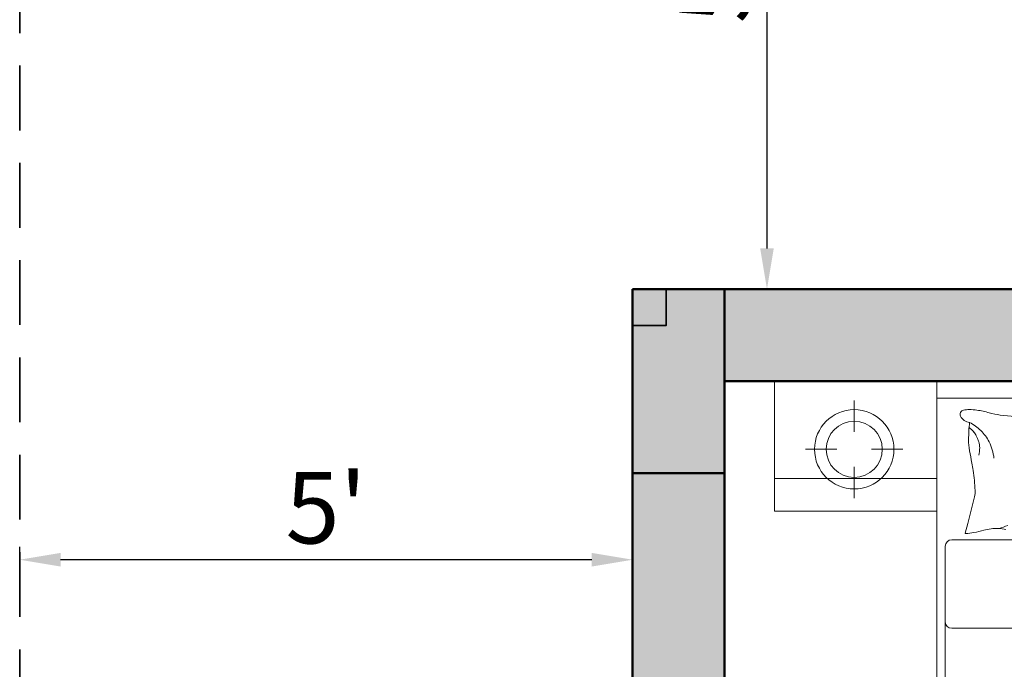
# Model space of a CAD drawing. Units: inches. Extents: x -7 to 1228, y -146 to 1091.
# Tile 53 of 88: x 0 to 96, y 964 to 1027. Entities that reach past the tile are written whole.
import ezdxf

# ---------------------------------------------------------------- set-up
doc = ezdxf.new("R2010")
doc.units = ezdxf.units.IN
doc.linetypes.add('DASHED2', pattern=[9.525, 6.35, -3.175])
for name, color, linetype, lineweight in [('A-ANNO-DIMS', 2, 'Continuous', 18), ('A-COLS', 6, 'Continuous', 35), ('A-FURN', 8, 'Continuous', 18), ('A-WALL', 7, 'Continuous', 50), ('A-WALL-PATT', 251, 'Continuous', 13), ('C-PROP', 1, 'DASHED2', 35)]:
    doc.layers.add(name, color=color, linetype=linetype, lineweight=lineweight)
doc.styles.add('DIM_FONT', font='SIMPLEX.shx', dxfattribs={"width": 0.8})
doc.styles.get("Standard").update_dxf_attribs({"font": 'arial.ttf'})
doc.dimstyles.new('ISO-25', dxfattribs={"dimtxt": 7, "dimasz": 4, "dimexe": 1.25, "dimexo": 0.625, "dimtad": 1, "dimdec": 1, "dimlunit": 3, "dimtxsty": 'Standard', "dimcen": 2.5, "dimadec": 0, "dimazin": 0, "dimtfac": 1, "dimtdec": 1, "dimtmove": 1, "dimatfit": 3, "dimfxl": 1, "dimarcsym": 0})

# ---------------------------------------------------------------- blocks, each defined once
blk = doc.blocks.new('A$C4F634EDD')
for p, q in [((0, 2.6295), (0, 2.2295)), ((0.5, 2.6295), (0, 2.6295)), ((0.5, 2.6295), (2.3, 2.6295)), ((0.5, 0.5295), (0.5, 2.6295)), ((0.5, 2.2295), (0.5, 2.6295)), ((0.2457, 2.5697), (0.2457, 2.4733)), ((0.5, 2.5771), (2.3, 2.5771)), ((0.0957, 2.4197), (0.192, 2.4197)), ((0.2994, 2.4197), (0.3957, 2.4197)), ((0.2457, 2.366), (0.2457, 2.2697)), ((0, 2.3301), (0.5, 2.3301)), ((0.5953, 2.1912), (0.616, 2.2738)), ((0, 2.2295), (0.5, 2.2295)), ((0.5878, 2.1612), (0.5953, 2.1912)), ((1.5035, 2.141), (0.5458, 2.141)), ((0.5258, 2.121), (0.5258, 0.5617)), ((0.5458, 1.8684), (1.5653, 1.8684))]:
    blk.add_line(p, q)
for radius in [0.1222, 0.0865]:
    blk.add_circle((0.2457, 2.4197), radius)
for centre, radius, start, end in [((0.5848, 2.5274), 0.0131, 101.2724, 206.5805), ((0.6036, 2.5368), 0.0342, 206.5805, 265.5998), ((0.5999, 2.4516), 0.0904, 90, 101.2724), ((0.5999, 2.3808), 0.1611, 81.5628, 90), ((0.5788, 2.2388), 0.3048, 74.256, 81.5628), ((0.7272, 2.7653), 0.2422, 254.256, 262.4531), ((0.7851, 3.2019), 0.6827, 262.4531, 270), ((1.0898, 2.4496), 0.4918, 173.7676, 180), ((0.5462, 2.4142), 0.0899, 41.4429, 53.7359), ((0.5368, 2.3783), 0.1399, 45.0976, 62.7964), ((0.5741, 2.4389), 0.0526, 25.3551, 41.4429), ((0.4851, 2.3967), 0.1511, 21.8149, 25.3551), ((0.5368, 2.3783), 0.1399, 27.3988, 45.0976), ((0.8019, 2.4496), 0.204, 180, 189.6844), ((0.4345, 2.3765), 0.2056, 18.7799, 21.8149), ((0.576, 2.4246), 0.0562, 0, 18.7799), ((0.5368, 2.3783), 0.1399, 16.515, 27.3988), ((1.4703, 2.5637), 0.882, 189.6844, 192.1984), ((0.5406, 2.4246), 0.0915, 345.3149, 0), ((0.5368, 2.3783), 0.1399, 5.6311, 16.515), ((0.2982, 2.3103), 0.3171, 8.0051, 12.1984), ((-0.0401, 2.2627), 0.6588, 2.6649, 8.0051), ((0.5503, 2.2902), 0.0677, 345.9548, 2.6649), ((0.473, 2.8815), 0.7387, 287.1982, 289.428), ((0.5887, 2.1609), 0.000917, 165.9551, 274.0829), ((0.5695, 2.4301), 0.2708, 274.0829, 279.4841), ((0.5763, 2.3896), 0.2297, 279.4841, 287.3864), ((0.6807, 2.0561), 0.1197, 96.4341, 107.3864), ((0.6836, 2.0301), 0.1459, 78.4414, 96.4341), ((0.5458, 2.121), 0.02, 90, 180), ((0.5458, 1.8884), 0.02, 180, 270)]:
    blk.add_arc(centre, radius, start, end)
at = {"style": 'DIM_FONT', "width": 0.8, "flags": 9}
for tag, p in [('YSIZE', (0.5, 2.6295)), ('XSIZE', (0.5, 2.6295)), ('XSIZE', (2.2985, 2.6295)), ('YSIZE', (2.2985, 2.6295))]:
    blk.add_attdef(tag, p, '', height=0.0005, dxfattribs=at)
blk = doc.blocks.new('*D14')
at = {"layer": 'A-ANNO-DIMS', "color": 0, "lineweight": -2, "transparency": 16777216}
for p, q in [((0, 975.149), (0, 975.774)), ((60, 975.149), (60, 975.774)), ((56, 974.524), (4, 974.524))]:
    blk.add_line(p, q, dxfattribs=at)
at = {"layer": 'A-ANNO-DIMS', "color": 0, "transparency": 16777216}
for points in [[(4, 975.19), (4, 973.857), (0, 974.524)], [(56, 975.19), (56, 973.857), (60, 974.524)]]:
    blk.add_solid(points, dxfattribs=at)
at = {"layer": 'Defpoints', "color": 0, "transparency": 16777216}
for p in [(0, 974.524), (0, 974.524), (60, 974.524)]:
    blk.add_point(p, dxfattribs=at)
at = {"layer": 'A-ANNO-DIMS', "color": 0, "transparency": 16777216, "insert": (30, 978.708), "char_height": 7, "attachment_point": 5}
blk.add_mtext("5'", dxfattribs=at)
blk = doc.blocks.new('*D15')
at = {"layer": 'A-ANNO-DIMS', "color": 0, "lineweight": -2, "transparency": 16777216}
for p, q in [((68.951, 1061), (74.399, 1061)), ((73.149, 1057), (73.149, 1005)), ((68.951, 1001), (74.399, 1001))]:
    blk.add_line(p, q, dxfattribs=at)
at = {"layer": 'A-ANNO-DIMS', "color": 0, "transparency": 16777216}
for points in [[(72.482, 1057), (73.815, 1057), (73.149, 1061)], [(72.482, 1005), (73.815, 1005), (73.149, 1001)]]:
    blk.add_solid(points, dxfattribs=at)
at = {"layer": 'Defpoints', "color": 0, "transparency": 16777216}
for p in [(68.326, 1061), (68.326, 1001), (73.149, 1001)]:
    blk.add_point(p, dxfattribs=at)
at = {"layer": 'A-ANNO-DIMS', "color": 0, "transparency": 16777216, "insert": (68.964, 1031), "char_height": 7, "attachment_point": 5, "rotation": 90}
blk.add_mtext("5'", dxfattribs=at)

msp = doc.modelspace()

# ---------------------------------------------------------------- hatches: boundary and pattern name
at = {"layer": 'A-COLS'}
h = msp.add_hatch(color=256, dxfattribs=at)
h.dxf.hatch_style = 1
h.paths.add_polyline_path([(60, 983), (69, 983), (69, 1001), (63.289, 1001), (63.289, 997.454), (60, 997.454)])
h = msp.add_hatch(color=256, dxfattribs=at)
h.dxf.hatch_style = 1
h.paths.add_polyline_path([(63.289, 997.454), (63.289, 1001), (60, 1001), (60, 997.454)])
at = {"layer": 'A-WALL-PATT'}
h = msp.add_hatch(color=256, dxfattribs=at)
h.dxf.hatch_style = 1
h.paths.add_polyline_path([(69, 568), (60, 568), (60, 493), (63.289, 493), (69, 493)])
h.paths.add_polyline_path([(69, 662.405), (60, 662.405), (60, 586), (69, 586)], flags=17)
h.paths.add_polyline_path([(69, 723), (184, 723), (184, 734), (179, 734), (179, 728), (69, 728), (69, 741.623), (60, 741.623), (60, 698.405), (69, 698.405)], flags=17)
h.paths.add_polyline_path([(69, 782), (231, 782), (231, 728), (231, 723), (231, 586), (236, 586), (236, 787), (69, 787), (69, 800.126), (60, 800.126), (60, 765.623), (69, 765.623)])
h.paths.add_polyline_path([(184, 842), (189, 842), (189, 848), (173, 848), (173, 842), (179, 842), (179, 787), (184, 787)])
h.paths.add_polyline_path([(118.22, 69), (69, 69), (69, 60), (118.22, 60)])
h.paths.add_polyline_path([(227, 69), (154.22, 69), (154.22, 60), (227, 60)])
h.paths.add_polyline_path([(236, 60), (232.711, 60), (227, 60), (227, 36), (236, 36)])
h.paths.add_polyline_path([(389, 60), (380, 60), (380, 36), (389, 36)])
h.paths.add_polyline_path([(384, 181), (380, 181), (380, 115), (380, 78), (384, 78)])
h.paths.add_polyline_path([(380, 115), (334.547, 115), (334.547, 109), (380, 109)])
h.paths.add_polyline_path([(274.547, 115), (236, 115), (236, 201), (232.711, 201), (231, 201), (231, 78), (236, 78), (236, 109), (274.547, 109)])
h.paths.add_polyline_path([(69, 123), (60, 123), (60, 78), (69, 78)])
h.paths.add_polyline_path([(69, 201), (60, 201), (60, 159), (69, 159)])
h.paths.add_polyline_path([(143, 219), (69, 219), (69, 213), (143, 213)], flags=17)
h.paths.add_polyline_path([(189, 219), (184, 219), (184, 274), (231, 274), (231, 219), (236, 219), (236, 279), (184, 279), (184, 297), (179, 297), (179, 279), (69, 279), (69, 290.912), (60, 290.912), (60, 262.179), (69, 262.179), (69, 274), (179, 274), (179, 219), (173, 219), (173, 213), (189, 213)])
h.paths.add_polyline_path([(69, 238.179), (60, 238.179), (60, 219), (69, 219)], flags=17)
h.paths.add_polyline_path([(69, 333), (60, 333), (60, 314.912), (69, 314.912), (69, 316.965)])
h.paths.add_polyline_path([(190, 338), (184, 338), (69, 338), (69, 333), (179, 333), (179, 327), (184, 327), (184, 333.021), (190, 333.046)])
h.paths.add_polyline_path([(69, 386.806), (60, 386.806), (60, 351), (69, 351)])
h.paths.add_polyline_path([(69, 475), (60, 475), (60, 422.806), (69, 422.806)])
h.paths.add_polyline_path([(236, 475), (231, 475), (231, 351.238), (236, 351.238)])
h.paths.add_polyline_path([(384, 475), (380, 475), (380, 362), (384, 362)])
h.paths.add_polyline_path([(547, 307), (439, 307), (439, 356), (445, 356), (445, 362), (433, 362), (433, 307), (380, 307), (380, 244), (380, 241), (384, 241), (384, 301), (433, 301), (433, 277), (439, 277), (439, 301), (547, 301)])
h.paths.add_polyline_path([(547, 241), (439, 241), (439, 247), (433, 247), (433, 235), (547, 235)])
h.paths.add_polyline_path([(450, 69), (440.286, 69), (424.889, 69), (389, 69), (389, 60), (450, 60)])
h.paths.add_polyline_path([(547, 69), (486, 69), (486, 60), (547, 60)])
h.paths.add_polyline_path([(556, 148.268), (547, 148.268), (547, 78), (556, 78)])
h.paths.add_polyline_path([(556, 223), (547, 223), (547, 195), (547, 184.268), (556, 184.268)])
h.paths.add_polyline_path([(556, 311.192), (547, 311.192), (547, 273.075), (556, 273.075)])
h.paths.add_polyline_path([(556, 344), (552.711, 344), (547, 344), (547, 335.192), (556, 335.192)])
h.paths.add_polyline_path([(556, 249.075), (547, 249.075), (547, 241), (556, 241)])
h.paths.add_polyline_path([(547, 362), (475, 362), (475, 356), (547, 356)], flags=0)
h.paths.add_polyline_path([(556, 399.621), (547, 399.621), (547, 362), (556, 362)])
h.paths.add_polyline_path([(556, 475), (547, 475), (547, 435.621), (556, 435.621)])
h.paths.add_polyline_path([(547, 493), (389, 493), (389, 487), (547, 487)])
h.paths.add_polyline_path([(380, 493), (278, 493), (278, 487), (380, 487)])
h.paths.add_polyline_path([(227, 493), (69, 493), (69, 487), (227, 487)])
h.paths.add_polyline_path([(643, 122.445), (634, 122.445), (634, 78), (643, 78)])
h.paths.add_polyline_path([(702.5, 69), (692.786, 69), (677.389, 69), (643, 69), (643, 60), (702.5, 60)])
h.paths.add_polyline_path([(798, 69), (738.5, 69), (738.5, 60), (798, 60)])
h.paths.add_polyline_path([(807, 60), (803.711, 60), (798, 60), (798, 36), (807, 36)])
h.paths.add_polyline_path([(807, 109), (846.751, 109), (846.751, 115), (807, 115), (807, 159), (802, 159), (802, 78), (807, 78)])
h.paths.add_polyline_path([(807, 201), (802, 201), (802, 195), (807, 195)])
h.paths.add_polyline_path([(643, 201), (634, 201), (634, 158.445), (643, 158.445)])
h.paths.add_polyline_path([(756, 225), (751, 225), (751, 219), (643, 219), (643, 213), (756, 213)])
h.paths.add_polyline_path([(643, 240.848), (634, 240.848), (634, 219), (643, 219)])
h.paths.add_polyline_path([(643, 274), (643, 288.629), (634, 288.629), (634, 264.848), (643, 264.848)])
h.paths.add_polyline_path([(802, 279), (756, 279), (756, 297), (751, 297), (751, 279), (643, 279), (643, 274), (751, 274), (751, 255), (756, 255), (756, 274), (802, 274)])
h.paths.add_polyline_path([(807, 333), (803.711, 333), (802, 333), (802, 279), (802, 274), (802, 219), (807, 219)])
h.paths.add_polyline_path([(956, 182), (951, 182), (951, 115), (906.751, 115), (906.751, 109), (951, 109), (951, 78), (956, 78)])
h.paths.add_polyline_path([(960, 60), (951, 60), (951, 36), (960, 36)])
h.paths.add_polyline_path([(1021, 69), (1005.781, 69), (960, 69), (960, 60), (1021, 60)])
h.paths.add_polyline_path([(956, 224), (951, 224), (951, 218), (956, 218)])
h.paths.add_polyline_path([(956, 302), (1004, 302), (1004, 278), (1010, 278), (1010, 302), (1118, 302), (1118, 290.809), (1127, 290.809), (1127, 326.968), (1118, 326.968), (1118, 320.966), (1118, 307), (1010, 307), (1010, 356), (1016, 356), (1016, 362), (1004, 362), (1004, 307), (951, 307), (951, 244), (951, 242), (954.289, 242), (956, 242)])
h.paths.add_polyline_path([(643, 333), (634, 333), (634, 312.629), (643, 312.629), (643, 316.965)])
h.paths.add_polyline_path([(756, 338), (643, 338), (643, 333), (751, 333), (751, 327), (756, 327)])
h.paths.add_polyline_path([(643, 388), (634, 388), (634, 351), (643, 351)])
h.paths.add_polyline_path([(807, 357), (802, 357), (802, 351), (807, 351)])
h.paths.add_polyline_path([(807, 475), (802, 475), (802, 393), (807, 393)])
h.paths.add_polyline_path([(643, 475), (634, 475), (634, 424), (643, 424)])
h.paths.add_polyline_path([(798, 493), (643, 493), (643, 487), (798, 487)])
h.paths.add_polyline_path([(634, 493), (556, 493), (556, 487), (634, 487)])
h.paths.add_polyline_path([(813, 493), (807, 493), (807, 487), (813, 487)])
h.paths.add_polyline_path([(951, 493), (849, 493), (849, 487), (951, 487)])
h.paths.add_polyline_path([(956, 484), (951, 484), (951, 374), (956, 374)])
h.paths.add_polyline_path([(1109, 493), (969, 493), (969, 487), (1109, 487)])
h.paths.add_polyline_path([(1127, 484), (1118, 484), (1118, 450.641), (1127, 450.641)])
h.paths.add_polyline_path([(1127, 414.641), (1118, 414.641), (1118, 365), (1127, 365)])
h.paths.add_polyline_path([(1109, 362), (1046, 362), (1046, 356), (1109, 356)], flags=17)
h.paths.add_polyline_path([(1127, 356), (1123.454, 356), (1118, 356), (1118, 350.968), (1127, 350.968)], flags=0)
h.paths.add_polyline_path([(1127, 266.809), (1118, 266.809), (1118, 262.361), (1118, 242), (1127, 242)], flags=17)
h.paths.add_polyline_path([(1118, 242), (1010, 242), (1010, 248), (1004, 248), (1004, 237), (1118, 237)])
h.paths.add_polyline_path([(1127, 224), (1118, 224), (1118, 170), (1127, 170)])
h.paths.add_polyline_path([(1127, 134), (1118, 134), (1118, 78), (1127, 78)])
h.paths.add_polyline_path([(1118, 69), (1057, 69), (1057, 60), (1118, 60)])
h.paths.add_polyline_path([(227, 571.546), (227, 574), (69, 574), (69, 568), (227, 568)])
h.paths.add_polyline_path([(380, 571.546), (380, 574), (278, 574), (278, 568), (380, 568)])
h.paths.add_polyline_path([(242, 574), (236, 574), (236, 568), (242, 568)])
h.paths.add_polyline_path([(547, 571.546), (547, 574), (389, 574), (389, 568), (547, 568)])
h.paths.add_polyline_path([(384, 733), (380, 733), (380, 586), (384, 586)])
h.paths.add_polyline_path([(556, 646), (634, 646), (634, 655), (547, 655), (547, 586), (556, 586)])
h.paths.add_polyline_path([(634, 574), (556, 574), (556, 568), (634, 568)])
h.paths.add_polyline_path([(643, 655), (634, 655), (634, 586), (643, 586)])
h.paths.add_polyline_path([(798, 574), (643, 574), (643, 568), (798, 568)])
h.paths.add_polyline_path([(643, 663.854), (634, 663.854), (634, 655), (643, 655)])
h.paths.add_polyline_path([(556, 676.967), (547, 676.967), (547, 655), (556, 655)])
h.paths.add_polyline_path([(556, 733), (547, 733), (547, 712.967), (556, 712.967)])
h.paths.add_polyline_path([(643, 710), (634, 710), (634, 699.854), (643, 699.854)])
h.paths.add_polyline_path([(807, 668), (802, 668), (802, 586), (807, 586)])
h.paths.add_polyline_path([(951, 574), (849, 574), (849, 568), (951, 568)])
h.paths.add_polyline_path([(956, 691), (951, 691), (951, 577), (956, 577)])
h.paths.add_polyline_path([(1109, 574), (969, 574), (969, 568), (1109, 568)])
h.paths.add_polyline_path([(1127, 643.403), (1118, 643.403), (1118, 577), (1127, 577)])
h.paths.add_polyline_path([(1127, 568), (1123.454, 568), (1118, 568), (1118, 493), (1127, 493)])
h.paths.add_polyline_path([(1127, 733), (1118, 733), (1118, 679.403), (1127, 679.403)])
h.paths.add_polyline_path([(1127, 777.348), (1118, 777.348), (1118, 770.035), (1118, 751), (1127, 751)], flags=17)
h.paths.add_polyline_path([(1118, 751), (1010, 751), (1010, 757), (1004, 757), (1004, 745), (1118, 745)])
h.paths.add_polyline_path([(956, 811), (1004, 811), (1004, 787), (1010, 787), (1010, 811), (1017.874, 811), (1017.874, 811.627, -0.414214), (1018.247, 812), (1031.978, 812, -0.414214), (1032.351, 811.627), (1032.351, 811), (1118, 811), (1118, 801.348), (1127, 801.348), (1127, 834.685), (1118, 834.685), (1118, 830.238), (1118, 817), (1010, 817), (1010, 866), (1016, 866), (1016, 872), (1004, 872), (1004, 817), (956, 817), (956, 866), (951, 866), (951, 751), (954.289, 751), (956, 751)])
h.paths.add_polyline_path([(1118, 872), (1046, 872), (1046, 866), (1118, 866)], flags=17)
h.paths.add_polyline_path([(1127, 924.711), (1118, 924.711), (1118, 884), (1127, 884)])
h.paths.add_polyline_path([(1127, 866), (1123.711, 866), (1118, 866), (1118, 858.685), (1127, 858.685)], flags=17)
h.paths.add_polyline_path([(956, 983), (951, 983), (951, 952), (807, 952), (807, 983), (802, 983), (802, 902), (807, 902), (807, 946), (951, 946), (951, 884), (956, 884)])
h.paths.add_polyline_path([(807, 842), (802, 842), (802, 787), (756, 787), (756, 806), (751, 806), (751, 787), (643, 787), (643, 782), (751, 782), (751, 764), (756, 764), (756, 782), (802, 782), (802, 728), (807, 728)])
h.paths.add_polyline_path([(756, 848), (643, 848), (643, 842), (751, 842), (751, 836), (756, 836)])
h.paths.add_polyline_path([(756, 734), (751, 734), (751, 728), (643, 728), (643, 723), (756, 723)])
h.paths.add_polyline_path([(643, 749.791), (634, 749.791), (634, 728), (637.289, 728), (643, 728)])
h.paths.add_polyline_path([(643, 805.405), (634, 805.405), (634, 773.791), (643, 773.791)])
h.paths.add_polyline_path([(643, 896.663), (634, 896.663), (634, 860), (637.289, 860), (643, 860)])
h.paths.add_polyline_path([(643, 842), (634, 842), (634, 829.405), (643, 829.405)])
h.paths.add_polyline_path([(643, 983), (634, 983), (634, 932.663), (643, 932.663)])
h.paths.add_polyline_path([(1127, 983), (1118, 983), (1118, 960.711), (1127, 960.711)])
h.paths.add_polyline_path([(1118, 1001), (1077.525, 1001), (1077.525, 992), (1118, 992)])
h.paths.add_polyline_path([(1041.525, 1001), (960, 1001), (960, 992), (1041.525, 992)])
h.paths.add_polyline_path([(960, 1025), (951, 1025), (951, 1001), (954.289, 1001), (960, 1001)])
h.paths.add_polyline_path([(807, 1025), (798, 1025), (798, 1001), (807, 1001)])
h.paths.add_polyline_path([(798, 1001), (738.5, 1001), (738.5, 992), (798, 992)])
h.paths.add_polyline_path([(702.5, 1001), (643, 1001), (643, 992), (702.5, 992)])
h.paths.add_polyline_path([(547, 1001), (499.113, 1001), (499.113, 992), (547, 992)])
h.paths.add_polyline_path([(463.113, 1001), (389, 1001), (389, 992), (463.113, 992)])
h.paths.add_polyline_path([(389, 1025), (380, 1025), (380, 1022), (380, 1001), (383.289, 1001), (389, 1001)])
h.paths.add_polyline_path([(236, 1025), (227, 1025), (227, 1001), (236, 1001)])
h.paths.add_polyline_path([(236, 983), (231, 983), (231, 860), (236, 860)])
h.paths.add_polyline_path([(274.547, 952), (236, 952), (236, 946), (274.547, 946)])
h.paths.add_polyline_path([(380, 952), (334.547, 952), (334.547, 946), (380, 946)])
h.paths.add_polyline_path([(384, 983), (380, 983), (380, 884), (383.289, 884), (384, 884)])
h.paths.add_polyline_path([(227, 1001), (155.012, 1001), (155.012, 992), (162.875, 992), (227, 992)])
h.paths.add_polyline_path([(119.012, 1001), (69, 1001), (69, 992), (119.012, 992)])
h.paths.add_polyline_path([(69, 983), (60, 983), (60, 922.987), (69, 922.987)])
h.paths.add_polyline_path([(69, 886.987), (60, 886.987), (60, 860), (63.289, 860), (69, 860)])
h.paths.add_polyline_path([(143, 848), (69, 848), (69, 842), (143, 842)])

# ---------------------------------------------------------------- linework, layer by layer
at = {"layer": 'A-COLS'}
msp.add_lwpolyline([(60, 1001), (63.289, 1001), (63.289, 997.454), (60, 997.454)], close=True, dxfattribs=at)
at = {"layer": 'A-WALL'}
for p, q in [((60, 1001), (60, 60)), ((236, 1001), (60, 1001)), ((60, 1001), (69, 1001)), ((60, 983), (60, 1001)), ((69, 1001), (69, 983)), ((69, 992), (69, 848)), ((231, 992), (69, 992)), ((69, 983), (60, 983))]:
    msp.add_line(p, q, dxfattribs=at)
at = {"layer": 'C-PROP'}
msp.add_line((0, 1061), (0, 0), dxfattribs=at)

# ---------------------------------------------------------------- block references
at = {"layer": 'A-FURN', "xscale": 31.78426361944092, "yscale": 31.78426361944092, "zscale": 31.78426361944092}
msp.add_blockref('A$C4F634EDD', (73.879, 908.423), dxfattribs=at)

# ---------------------------------------------------------------- dimensions: what is measured, and where the dimension line sits
at = {"layer": 'A-ANNO-DIMS'}
dim = msp.add_linear_dim(base=(73.149, 1001), p1=(68.326, 1061), p2=(68.326, 1001), angle=90, dimstyle='ISO-25', override={"dimclrd": 0, "dimclre": 0, "dimclrt": 0}, dxfattribs=at)
dim.commit()
dim.dimension.update_dxf_attribs({"geometry": '*D15', "text_midpoint": (68.964, 1031)})
dim = msp.add_linear_dim(base=(0, 974.524), p1=(60, 974.524), p2=(0, 974.524), dimstyle='ISO-25', override={"dimclrd": 0, "dimclre": 0, "dimclrt": 0}, dxfattribs=at)
dim.commit()
dim.dimension.update_dxf_attribs({"geometry": '*D14', "text_midpoint": (30, 978.708)})

doc.saveas('drawing.dxf')
